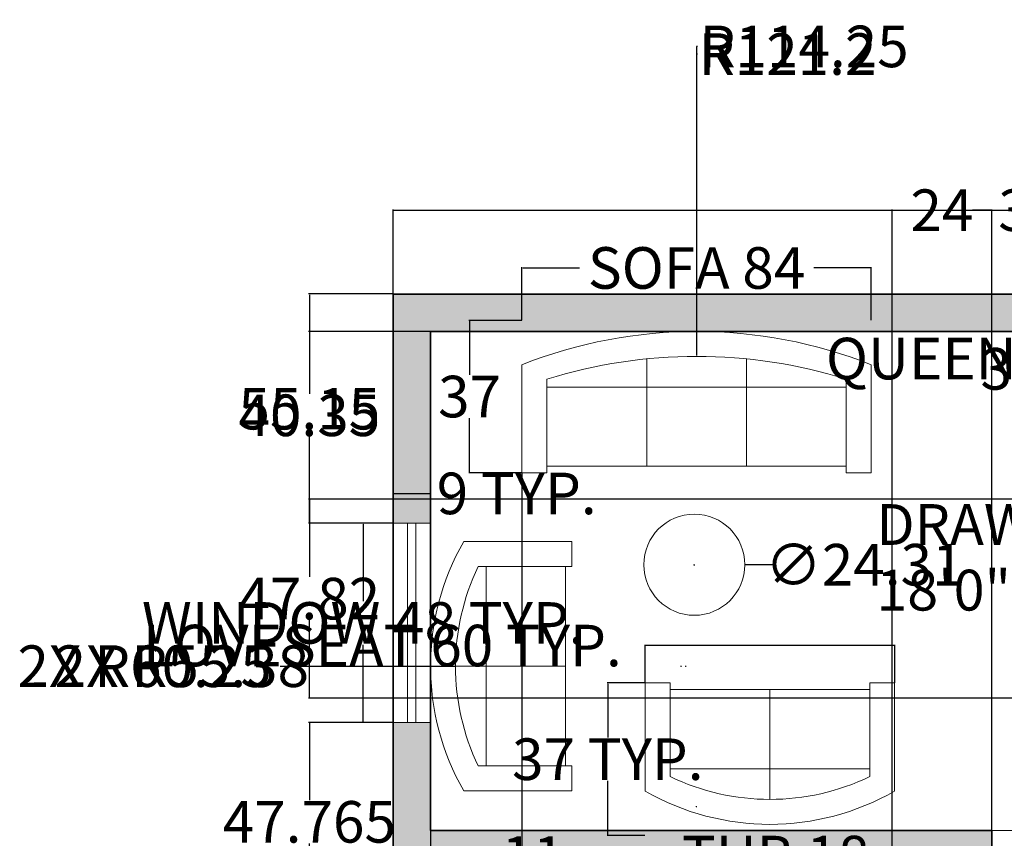
# Model space of a CAD drawing. Units: inches. Extents: x -75 to 484, y -248 to 214.
# Tile 3 of 7: x -75 to 162, y 17 to 214. Entities that reach past the tile are written whole.
import ezdxf

# ---------------------------------------------------------------- set-up
doc = ezdxf.new("R2010")
doc.units = ezdxf.units.IN
doc.header["$MEASUREMENT"] = 0
doc.linetypes.add('ACAD_ISO02W100', pattern=[15, 12, -3])
for name, color, linetype, lineweight in [('A-ANNO-DIMS', 2, 'Continuous', 18), ('A-AREA-IDEN', 7, 'Continuous', 18), ('A-FURN', 8, 'Continuous', 18), ('A-GLAZ', 4, 'Continuous', 18), ('A-WALL', 7, 'Continuous', 35), ('A-WALL-OVHD', 7, 'ACAD_ISO02W100', 18)]:
    doc.layers.add(name, color=color, linetype=linetype, lineweight=lineweight)
doc.layers.add('A-WALL-PATT', color=252, linetype='Continuous', lineweight=9, true_color=0x939598)
doc.styles.get("Standard").update_dxf_attribs({"font": 'arial.ttf'})
doc.dimstyles.get("Standard").update_dxf_attribs({"dimtxt": 10, "dimasz": 0.18, "dimexe": 0.18, "dimexo": 0.0625, "dimgap": 0.09, "dimtad": 0, "dimtih": 1, "dimtoh": 1, "dimdec": 0, "dimzin": 0, "dimdsep": 46, "dimlunit": 3, "dimtxsty": 'Standard', "dimcen": 0.09, "dimadec": 0, "dimazin": 0, "dimtfac": 1, "dimtdec": 0, "dimtofl": 0, "dimtmove": 0, "dimatfit": 3, "dimfxl": 1, "dimtolj": 1, "dimtzin": 0, "dimarcsym": 0})

# ---------------------------------------------------------------- blocks, each defined once
blk = doc.blocks.new('Sofa - Roundback 7 ft.')
for p, q in [((-12.00002, -32.4421), (-12.00003, -6.5971)), ((11.99997, -32.4421), (11.99998, -6.5971)), ((-36.000027, -34), (-36.000027, -11.4696)), ((35.99998, -34), (35.99998, -11.4696)), ((-35.999844, -13.3819), (35.9998, -13.3819)), ((-36.000027, -32.4421), (35.99998, -32.4421))]:
    blk.add_line(p, q)
for points in [[(-36.000027, -34), (-42.000027, -34), (-42.000027, -8)], [(41.99998, -8), (41.99998, -34), (35.99998, -34)]]:
    blk.add_lwpolyline(points)
for centre, radius, start, end in [((0, -114.25), 114.25, 68.43141, 111.5686), ((-0.00001, -127.1968), 121.1968, 72.72033, 107.2797)]:
    blk.add_arc(centre, radius, start, end)
blk = doc.blocks.new('Sofa - Roundback Loveseat 5 ft.')
for p, q in [((0, -32.44198), (0, -5.99998)), ((-24, -33.99998), (-24, -11.46958)), ((24.00004, -33.99998), (24.00004, -11.46958)), ((-23.9998, -13.38178), (23.99986, -13.38178)), ((-24, -32.44198), (24.00004, -32.44198))]:
    blk.add_line(p, q)
for points in [[(-24, -33.99998), (-30, -33.99998), (-30, -7.99998)], [(30.00004, -7.99998), (30.00004, -33.99998), (24.00004, -33.99998)]]:
    blk.add_lwpolyline(points)
for centre, radius, start, end in [((0, -60.24998), 60.24998, 60.13715, 119.8628), ((0, -61.38438), 55.38444, 64.32083, 115.6792)]:
    blk.add_arc(centre, radius, start, end)
blk = doc.blocks.new('WIN-48-NOM')
for p, q in [((9, 47.92), (0, 47.92)), ((3.5, 0), (3.5, 47.92)), ((5.5, 0), (5.5, 47.92)), ((0, 0), (9, 0))]:
    blk.add_line(p, q)
blk = doc.blocks.new('*D14')
at = {"layer": 'A-ANNO-DIMS', "color": 0, "lineweight": -2, "transparency": 16777216}
for p, q in [((184.84, 147.66), (179.32, 147.66)), ((179.5, 147.48), (179.5, 134.86)), ((179.5, 111.84), (179.5, 124.46)), ((184.84, 111.66), (179.32, 111.66))]:
    blk.add_line(p, q, dxfattribs=at)
at = {"layer": 'A-ANNO-DIMS', "color": 0, "transparency": 16777216}
for points in [[(179.47, 147.48), (179.53, 147.48), (179.5, 147.66)], [(179.47, 111.84), (179.53, 111.84), (179.5, 111.66)]]:
    blk.add_solid(points, dxfattribs=at)
at = {"layer": 'Defpoints', "color": 0, "transparency": 16777216}
for p in [(179.5, 147.66), (184.9, 147.66), (184.9, 111.66)]:
    blk.add_point(p, dxfattribs=at)
at = {"layer": 'A-ANNO-DIMS', "color": 0, "transparency": 16777216, "insert": (179.5, 129.66), "char_height": 10, "attachment_point": 5}
blk.add_mtext('\\A1;36 TYP.', dxfattribs=at)
blk = doc.blocks.new('*D17')
at = {"layer": 'A-ANNO-DIMS', "color": 0, "lineweight": -2, "transparency": 16777216}
for p, q in [((15.15, 92.5), (7.84, 92.5)), ((8.02, 92.32), (8.02, 73.81)), ((8.02, 44.77), (8.02, 63.28)), ((15.15, 44.59), (7.84, 44.59))]:
    blk.add_line(p, q, dxfattribs=at)
at = {"layer": 'A-ANNO-DIMS', "color": 0, "transparency": 16777216}
for points in [[(7.99, 92.32), (8.05, 92.32), (8.02, 92.5)], [(7.99, 44.77), (8.05, 44.77), (8.02, 44.59)]]:
    blk.add_solid(points, dxfattribs=at)
at = {"layer": 'Defpoints', "color": 0, "transparency": 16777216}
for p in [(8.02, 92.5), (15.21, 92.5), (15.21, 44.59)]:
    blk.add_point(p, dxfattribs=at)
at = {"layer": 'A-ANNO-DIMS', "color": 0, "transparency": 16777216, "insert": (8.02, 68.54), "char_height": 10, "attachment_point": 5}
blk.add_mtext('\\A1;WINDOW 48 TYP.', dxfattribs=at)
blk = doc.blocks.new('*D18')
at = {"layer": 'A-ANNO-DIMS', "color": 0, "lineweight": -2, "transparency": 16777216}
for p, q in [((15.21, 92.57), (15.21, 99.87)), ((15.39, 99.69), (24.03, 99.69)), ((24.21, 92.57), (24.21, 99.87)), ((24.21, 99.69), (24.39, 99.69))]:
    blk.add_line(p, q, dxfattribs=at)
at = {"layer": 'A-ANNO-DIMS', "color": 0, "transparency": 16777216}
for points in [[(15.39, 99.72), (15.39, 99.66), (15.21, 99.69)], [(24.03, 99.72), (24.03, 99.66), (24.21, 99.69)]]:
    blk.add_solid(points, dxfattribs=at)
at = {"layer": 'Defpoints', "color": 0, "transparency": 16777216}
for p in [(24.21, 99.69), (15.21, 92.5), (24.21, 92.5)]:
    blk.add_point(p, dxfattribs=at)
at = {"layer": 'A-ANNO-DIMS', "color": 0, "transparency": 16777216, "insert": (44.93, 99.69), "char_height": 10, "attachment_point": 5}
blk.add_mtext('\\A1;9 TYP.', dxfattribs=at)
blk = doc.blocks.new('*D19')
at = {"layer": 'A-ANNO-DIMS', "color": 0, "lineweight": -2, "transparency": 16777216}
for p, q in [((249.21, 132.13), (249.03, 132.13)), ((249.21, 120.19), (249.21, 132.31)), ((329.03, 132.13), (249.39, 132.13)), ((329.21, 120.19), (329.21, 132.31))]:
    blk.add_line(p, q, dxfattribs=at)
at = {"layer": 'A-ANNO-DIMS', "color": 0, "transparency": 16777216}
for points in [[(249.39, 132.16), (249.39, 132.1), (249.21, 132.13)], [(329.03, 132.16), (329.03, 132.1), (329.21, 132.13)]]:
    blk.add_solid(points, dxfattribs=at)
at = {"layer": 'Defpoints', "color": 0, "transparency": 16777216}
for p in [(249.21, 132.13), (249.21, 120.13), (329.21, 120.13)]:
    blk.add_point(p, dxfattribs=at)
at = {"layer": 'A-ANNO-DIMS', "color": 0, "transparency": 16777216, "insert": (181.53, 132.13), "char_height": 10, "attachment_point": 5}
blk.add_mtext('\\A1;QUEEN BED 80 TYP.', dxfattribs=at)
blk = doc.blocks.new('*D23')
at = {"layer": 'A-ANNO-DIMS', "color": 0, "lineweight": -2, "transparency": 16777216}
for p, q in [((75.84, 63.1), (75.66, 63.1)), ((75.84, 54.16), (75.84, 63.28)), ((135.66, 63.1), (76.02, 63.1)), ((135.84, 54.16), (135.84, 63.28))]:
    blk.add_line(p, q, dxfattribs=at)
at = {"layer": 'A-ANNO-DIMS', "color": 0, "transparency": 16777216}
for points in [[(76.02, 63.13), (76.02, 63.07), (75.84, 63.1)], [(135.66, 63.13), (135.66, 63.07), (135.84, 63.1)]]:
    blk.add_solid(points, dxfattribs=at)
at = {"layer": 'Defpoints', "color": 0, "transparency": 16777216}
for p in [(75.84, 63.1), (75.84, 54.1), (135.84, 54.1)]:
    blk.add_point(p, dxfattribs=at)
at = {"layer": 'A-ANNO-DIMS', "color": 0, "transparency": 16777216, "insert": (12.63, 63.1), "char_height": 10, "attachment_point": 5}
blk.add_mtext('\\A1;LOVESEAT 60 TYP.', dxfattribs=at)
blk = doc.blocks.new('*D24')
at = {"layer": 'A-ANNO-DIMS', "color": 0, "lineweight": -2, "transparency": 16777216}
for p, q in [((75.77, 54.1), (66.66, 54.1)), ((66.84, 53.92), (66.84, 40.97)), ((66.84, 17.61), (66.84, 30.57)), ((75.77, 17.43), (66.66, 17.43))]:
    blk.add_line(p, q, dxfattribs=at)
at = {"layer": 'A-ANNO-DIMS', "color": 0, "transparency": 16777216}
for points in [[(66.81, 53.92), (66.87, 53.92), (66.84, 54.1)], [(66.81, 17.61), (66.87, 17.61), (66.84, 17.43)]]:
    blk.add_solid(points, dxfattribs=at)
at = {"layer": 'Defpoints', "color": 0, "transparency": 16777216}
for p in [(75.84, 54.1), (66.84, 17.43), (75.84, 17.43)]:
    blk.add_point(p, dxfattribs=at)
at = {"layer": 'A-ANNO-DIMS', "color": 0, "transparency": 16777216, "insert": (66.84, 35.77), "char_height": 10, "attachment_point": 5}
blk.add_mtext('\\A1;37 TYP.', dxfattribs=at)
blk = doc.blocks.new('*D25')
at = {"layer": 'A-ANNO-DIMS', "color": 0, "lineweight": -2, "transparency": 16777216}
for p, q in [((46.2, 141.39), (46.2, 154.1)), ((130.2, 141.39), (130.2, 154.1)), ((46.38, 153.92), (60.03, 153.92)), ((130.02, 153.92), (116.37, 153.92))]:
    blk.add_line(p, q, dxfattribs=at)
at = {"layer": 'A-ANNO-DIMS', "color": 0, "transparency": 16777216}
for points in [[(46.38, 153.95), (46.38, 153.89), (46.2, 153.92)], [(130.02, 153.95), (130.02, 153.89), (130.2, 153.92)]]:
    blk.add_solid(points, dxfattribs=at)
at = {"layer": 'Defpoints', "color": 0, "transparency": 16777216}
for p in [(130.2, 153.92), (46.2, 141.32), (130.2, 141.32)]:
    blk.add_point(p, dxfattribs=at)
at = {"layer": 'A-ANNO-DIMS', "color": 0, "transparency": 16777216, "insert": (88.2, 153.92), "char_height": 10, "attachment_point": 5}
blk.add_mtext('\\A1;SOFA 84', dxfattribs=at)
blk = doc.blocks.new('*D26')
at = {"layer": 'A-ANNO-DIMS', "color": 0, "lineweight": -2, "transparency": 16777216}
for p, q in [((46.14, 141.32), (33.42, 141.32)), ((33.6, 141.14), (33.6, 128.19)), ((33.6, 104.84), (33.6, 117.79)), ((46.14, 104.66), (33.42, 104.66))]:
    blk.add_line(p, q, dxfattribs=at)
at = {"layer": 'A-ANNO-DIMS', "color": 0, "transparency": 16777216}
for points in [[(33.57, 141.14), (33.63, 141.14), (33.6, 141.32)], [(33.57, 104.84), (33.63, 104.84), (33.6, 104.66)]]:
    blk.add_solid(points, dxfattribs=at)
at = {"layer": 'Defpoints', "color": 0, "transparency": 16777216}
for p in [(33.6, 141.32), (46.2, 141.32), (46.2, 104.66)]:
    blk.add_point(p, dxfattribs=at)
at = {"layer": 'A-ANNO-DIMS', "color": 0, "transparency": 16777216, "insert": (33.6, 122.99), "char_height": 10, "attachment_point": 5}
blk.add_mtext('\\A1;37', dxfattribs=at)
blk = doc.blocks.new('*D30')
at = {"layer": 'A-ANNO-DIMS', "color": 0, "lineweight": -2, "transparency": 16777216}
for p, q in [((31.92, 9.72), (31.92, 12.43)), ((32.1, 12.25), (42.73, 12.25)), ((42.91, 9.72), (42.91, 12.43)), ((42.91, 12.25), (43.09, 12.25))]:
    blk.add_line(p, q, dxfattribs=at)
at = {"layer": 'A-ANNO-DIMS', "color": 0, "transparency": 16777216}
for points in [[(32.1, 12.28), (32.1, 12.22), (31.92, 12.25)], [(42.73, 12.28), (42.73, 12.22), (42.91, 12.25)]]:
    blk.add_solid(points, dxfattribs=at)
at = {"layer": 'Defpoints', "color": 0, "transparency": 16777216}
for p in [(42.91, 12.25), (31.92, 9.66), (42.91, 9.66)]:
    blk.add_point(p, dxfattribs=at)
at = {"layer": 'A-ANNO-DIMS', "color": 0, "transparency": 16777216, "insert": (48.9, 12.25), "char_height": 10, "attachment_point": 5}
blk.add_mtext('\\A1;11', dxfattribs=at)
blk = doc.blocks.new('*D33')
at = {"layer": 'A-ANNO-DIMS', "color": 0, "lineweight": -2, "transparency": 16777216}
for p, q in [((65.81, 9.72), (65.81, 12.53)), ((65.99, 12.35), (83.56, 12.35)), ((83.74, 9.72), (83.74, 12.53)), ((83.74, 12.35), (83.92, 12.35))]:
    blk.add_line(p, q, dxfattribs=at)
at = {"layer": 'A-ANNO-DIMS', "color": 0, "transparency": 16777216}
for points in [[(65.99, 12.38), (65.99, 12.32), (65.81, 12.35)], [(83.56, 12.38), (83.56, 12.32), (83.74, 12.35)]]:
    blk.add_solid(points, dxfattribs=at)
at = {"layer": 'Defpoints', "color": 0, "transparency": 16777216}
for p in [(83.74, 12.35), (65.81, 9.66), (83.74, 9.66)]:
    blk.add_point(p, dxfattribs=at)
at = {"layer": 'A-ANNO-DIMS', "color": 0, "transparency": 16777216, "insert": (107.22, 12.35), "char_height": 10, "attachment_point": 5}
blk.add_mtext('\\A1;TUB 18', dxfattribs=at)
blk = doc.blocks.new('*D41')
at = {"layer": 'A-ANNO-DIMS', "color": 0, "lineweight": -2, "transparency": 16777216}
for p, q in [((15.21, 147.72), (15.21, 167.99)), ((15.39, 167.81), (203.57, 167.81)), ((414.03, 167.81), (225.85, 167.81)), ((414.21, 147.72), (414.21, 167.99))]:
    blk.add_line(p, q, dxfattribs=at)
at = {"layer": 'A-ANNO-DIMS', "color": 0, "transparency": 16777216}
for points in [[(15.39, 167.84), (15.39, 167.78), (15.21, 167.81)], [(414.03, 167.84), (414.03, 167.78), (414.21, 167.81)]]:
    blk.add_solid(points, dxfattribs=at)
at = {"layer": 'Defpoints', "color": 0, "transparency": 16777216}
for p in [(414.21, 167.81), (15.21, 147.66), (414.21, 147.66)]:
    blk.add_point(p, dxfattribs=at)
at = {"layer": 'A-ANNO-DIMS', "color": 0, "transparency": 16777216, "insert": (214.71, 167.81), "char_height": 10, "attachment_point": 5}
blk.add_mtext('\\A1;399', dxfattribs=at)
blk = doc.blocks.new('*D44')
at = {"layer": 'A-ANNO-DIMS', "color": 0, "lineweight": -2, "transparency": 16777216}
for p, q in [((15.15, 147.66), (-5.12, 147.66)), ((-4.94, 147.48), (-4.94, 125.28)), ((-4.94, 92.68), (-4.94, 114.88)), ((15.15, 92.5), (-5.12, 92.5))]:
    blk.add_line(p, q, dxfattribs=at)
at = {"layer": 'A-ANNO-DIMS', "color": 0, "transparency": 16777216}
for points in [[(-4.97, 147.48), (-4.91, 147.48), (-4.94, 147.66)], [(-4.97, 92.68), (-4.91, 92.68), (-4.94, 92.5)]]:
    blk.add_solid(points, dxfattribs=at)
at = {"layer": 'Defpoints', "color": 0, "transparency": 16777216}
for p in [(15.21, 147.66), (-4.94, 92.5), (15.21, 92.5)]:
    blk.add_point(p, dxfattribs=at)
at = {"layer": 'A-ANNO-DIMS', "color": 0, "transparency": 16777216, "insert": (-4.94, 120.08), "char_height": 10, "attachment_point": 5}
blk.add_mtext('\\A1;55.15', dxfattribs=at)
blk = doc.blocks.new('*D45')
at = {"layer": 'A-ANNO-DIMS', "color": 0, "lineweight": -2, "transparency": 16777216}
for p, q in [((15.15, 44.59), (-5.12, 44.59)), ((-4.94, 44.41), (-4.94, 25.9)), ((-4.94, -3), (-4.94, 15.51)), ((15.15, -3.18), (-5.12, -3.18))]:
    blk.add_line(p, q, dxfattribs=at)
at = {"layer": 'A-ANNO-DIMS', "color": 0, "transparency": 16777216}
for points in [[(-4.97, 44.41), (-4.91, 44.41), (-4.94, 44.59)], [(-4.97, -3), (-4.91, -3), (-4.94, -3.18)]]:
    blk.add_solid(points, dxfattribs=at)
at = {"layer": 'Defpoints', "color": 0, "transparency": 16777216}
for p in [(15.21, 44.59), (-4.94, -3.18), (15.21, -3.18)]:
    blk.add_point(p, dxfattribs=at)
at = {"layer": 'A-ANNO-DIMS', "color": 0, "transparency": 16777216, "insert": (-4.94, 20.7), "char_height": 10, "attachment_point": 5}
blk.add_mtext('\\A1;47.765', dxfattribs=at)
blk = doc.blocks.new('*D50')
at = {"layer": 'A-ANNO-DIMS', "color": 0, "lineweight": -2, "transparency": 16777216}
for p, q in [((405.15, 138.66), (-5.12, 138.66)), ((-4.94, 138.48), (-4.94, 123.68)), ((-4.94, 98.48), (-4.94, 113.28)), ((405.15, 98.3), (-5.12, 98.3))]:
    blk.add_line(p, q, dxfattribs=at)
at = {"layer": 'A-ANNO-DIMS', "color": 0, "transparency": 16777216}
for points in [[(-4.97, 138.48), (-4.91, 138.48), (-4.94, 138.66)], [(-4.97, 98.48), (-4.91, 98.48), (-4.94, 98.3)]]:
    blk.add_solid(points, dxfattribs=at)
at = {"layer": 'Defpoints', "color": 0, "transparency": 16777216}
for p in [(405.21, 138.66), (-4.94, 98.3), (405.21, 98.3)]:
    blk.add_point(p, dxfattribs=at)
at = {"layer": 'A-ANNO-DIMS', "color": 0, "transparency": 16777216, "insert": (-4.94, 118.48), "char_height": 10, "attachment_point": 5}
blk.add_mtext('\\A1;40.35', dxfattribs=at)
blk = doc.blocks.new('*D51')
at = {"layer": 'A-ANNO-DIMS', "color": 0, "lineweight": -2, "transparency": 16777216}
for p, q in [((405.15, 98.3), (-5.12, 98.3)), ((-4.94, 98.12), (-4.94, 79.59)), ((-4.94, 50.66), (-4.94, 69.2)), ((405.15, 50.48), (-5.12, 50.48))]:
    blk.add_line(p, q, dxfattribs=at)
at = {"layer": 'A-ANNO-DIMS', "color": 0, "transparency": 16777216}
for points in [[(-4.97, 98.12), (-4.91, 98.12), (-4.94, 98.3)], [(-4.97, 50.66), (-4.91, 50.66), (-4.94, 50.48)]]:
    blk.add_solid(points, dxfattribs=at)
at = {"layer": 'Defpoints', "color": 0, "transparency": 16777216}
for p in [(405.21, 98.3), (-4.94, 50.48), (405.21, 50.48)]:
    blk.add_point(p, dxfattribs=at)
at = {"layer": 'A-ANNO-DIMS', "color": 0, "transparency": 16777216, "insert": (-4.94, 74.39), "char_height": 10, "attachment_point": 5}
blk.add_mtext('\\A1;47.82', dxfattribs=at)
blk = doc.blocks.new('*D54')
at = {"layer": 'A-ANNO-DIMS', "color": 0, "lineweight": -2, "transparency": 16777216}
for p, q in [((135.21, -50.28), (135.21, 167.99)), ((135.39, 167.81), (139.89, 167.81)), ((159.03, 167.81), (154.53, 167.81)), ((159.21, -50.28), (159.21, 167.99))]:
    blk.add_line(p, q, dxfattribs=at)
at = {"layer": 'A-ANNO-DIMS', "color": 0, "transparency": 16777216}
for points in [[(135.39, 167.84), (135.39, 167.78), (135.21, 167.81)], [(159.03, 167.84), (159.03, 167.78), (159.21, 167.81)]]:
    blk.add_solid(points, dxfattribs=at)
at = {"layer": 'Defpoints', "color": 0, "transparency": 16777216}
for p in [(159.21, 167.81), (135.21, -50.34), (159.21, -50.34)]:
    blk.add_point(p, dxfattribs=at)
at = {"layer": 'A-ANNO-DIMS', "color": 0, "transparency": 16777216, "insert": (147.21, 167.81), "char_height": 10, "attachment_point": 5}
blk.add_mtext('\\A1;24', dxfattribs=at)
blk = doc.blocks.new('*D76')
at = {"layer": 'A-ANNO-DIMS', "color": 0, "lineweight": -2, "transparency": 16777216}
for p, q in [((24.21, 138.59), (24.21, -241.67)), ((46.2, 104.59), (46.2, -241.67)), ((24.39, -241.49), (46.02, -241.49)), ((46.2, -241.49), (46.38, -241.49))]:
    blk.add_line(p, q, dxfattribs=at)
at = {"layer": 'A-ANNO-DIMS', "color": 0, "transparency": 16777216}
for points in [[(24.39, -241.46), (24.39, -241.52), (24.21, -241.49)], [(46.02, -241.46), (46.02, -241.52), (46.2, -241.49)]]:
    blk.add_solid(points, dxfattribs=at)
at = {"layer": 'Defpoints', "color": 0, "transparency": 16777216}
for p in [(24.21, 138.66), (46.2, 104.66), (46.2, -241.49)]:
    blk.add_point(p, dxfattribs=at)
at = {"layer": 'A-ANNO-DIMS', "color": 0, "transparency": 16777216, "insert": (63.44, -241.49), "char_height": 10, "attachment_point": 5}
blk.add_mtext('\\A1;21.99', dxfattribs=at)
blk = doc.blocks.new('*D77')
at = {"layer": 'A-ANNO-DIMS', "color": 0, "lineweight": -2, "transparency": 16777216}
for p, q in [((159.21, -53.28), (159.21, 167.99)), ((159.39, 167.81), (160.83, 167.81)), ((196.22, 167.81), (194.77, 167.81)), ((196.4, -54.9), (196.4, 167.99))]:
    blk.add_line(p, q, dxfattribs=at)
at = {"layer": 'A-ANNO-DIMS', "color": 0, "transparency": 16777216}
for points in [[(159.39, 167.84), (159.39, 167.78), (159.21, 167.81)], [(196.22, 167.84), (196.22, 167.78), (196.4, 167.81)]]:
    blk.add_solid(points, dxfattribs=at)
at = {"layer": 'Defpoints', "color": 0, "transparency": 16777216}
for p in [(196.4, 167.81), (159.21, -53.34), (196.4, -54.96)]:
    blk.add_point(p, dxfattribs=at)
at = {"layer": 'A-ANNO-DIMS', "color": 0, "transparency": 16777216, "insert": (177.8, 167.81), "char_height": 10, "attachment_point": 5}
blk.add_mtext('\\A1;37.19', dxfattribs=at)
blk = doc.blocks.new('*D81')
at = {"layer": 'A-ANNO-DIMS', "color": 0, "lineweight": -2, "transparency": 16777216}
for p, q in [((159.21, 18.72), (159.21, 167.99)), ((159.39, 167.81), (193.42, 167.81)), ((240.03, 167.81), (206, 167.81)), ((240.21, 18.72), (240.21, 167.99))]:
    blk.add_line(p, q, dxfattribs=at)
at = {"layer": 'A-ANNO-DIMS', "color": 0, "transparency": 16777216}
for points in [[(159.39, 167.84), (159.39, 167.78), (159.21, 167.81)], [(240.03, 167.84), (240.03, 167.78), (240.21, 167.81)]]:
    blk.add_solid(points, dxfattribs=at)
at = {"layer": 'Defpoints', "color": 0, "transparency": 16777216}
for p in [(240.21, 167.81), (159.21, 18.66), (240.21, 18.66)]:
    blk.add_point(p, dxfattribs=at)
at = {"layer": 'A-ANNO-DIMS', "color": 0, "transparency": 16777216, "insert": (199.71, 167.81), "char_height": 10, "attachment_point": 5}
blk.add_mtext('\\A1;81', dxfattribs=at)
blk = doc.blocks.new('*D83')
at = {"layer": 'A-ANNO-DIMS', "color": 0, "lineweight": -2, "transparency": 16777216}
for p, q in [((87.56, 82.54), (87.74, 82.54)), ((87.65, 82.45), (87.65, 82.63)), ((107.1, 82.54), (99.99, 82.54))]:
    blk.add_line(p, q, dxfattribs=at)
at = {"layer": 'A-ANNO-DIMS', "color": 0, "transparency": 16777216}
blk.add_solid([(99.99, 82.57), (99.99, 82.51), (99.81, 82.54)], dxfattribs=at)
at = {"layer": 'Defpoints', "color": 0, "transparency": 16777216}
for p in [(75.5, 82.54), (99.81, 82.54)]:
    blk.add_point(p, dxfattribs=at)
at = {"layer": 'A-ANNO-DIMS', "color": 0, "transparency": 16777216, "insert": (128.54, 82.54), "char_height": 10, "attachment_point": 5}
blk.add_mtext('\\A1;∅24.31', dxfattribs=at)
blk = doc.blocks.new('*D84')
at = {"layer": 'A-ANNO-DIMS', "color": 0, "lineweight": -2, "transparency": 16777216}
for p, q in [((88.38, 205.37), (88.2, 205.37)), ((88.2, 205.37), (88.2, 132.84)), ((88.11, 11.46), (88.29, 11.46)), ((88.2, 11.37), (88.2, 11.55))]:
    blk.add_line(p, q, dxfattribs=at)
at = {"layer": 'A-ANNO-DIMS', "color": 0, "transparency": 16777216}
blk.add_solid([(88.17, 132.84), (88.23, 132.84), (88.2, 132.66)], dxfattribs=at)
at = {"layer": 'Defpoints', "color": 0, "transparency": 16777216}
for p in [(88.2, 132.66), (88.2, 11.46)]:
    blk.add_point(p, dxfattribs=at)
at = {"layer": 'A-ANNO-DIMS', "color": 0, "transparency": 16777216, "insert": (110.08, 205.37), "char_height": 10, "attachment_point": 5}
blk.add_mtext('\\A1;R121.2', dxfattribs=at)
blk = doc.blocks.new('*D85')
at = {"layer": 'A-ANNO-DIMS', "color": 0, "lineweight": -2, "transparency": 16777216}
for p, q in [((88.38, 207.21), (88.2, 207.21)), ((88.2, 207.21), (88.2, 138.84)), ((88.11, 24.41), (88.29, 24.41)), ((88.2, 24.32), (88.2, 24.5))]:
    blk.add_line(p, q, dxfattribs=at)
at = {"layer": 'A-ANNO-DIMS', "color": 0, "transparency": 16777216}
blk.add_solid([(88.17, 138.84), (88.23, 138.84), (88.2, 138.66)], dxfattribs=at)
at = {"layer": 'Defpoints', "color": 0, "transparency": 16777216}
for p in [(88.2, 138.66), (88.2, 24.41)]:
    blk.add_point(p, dxfattribs=at)
at = {"layer": 'A-ANNO-DIMS', "color": 0, "transparency": 16777216, "insert": (114.05, 207.21), "char_height": 10, "attachment_point": 5}
blk.add_mtext('\\A1;R114.25', dxfattribs=at)
blk = doc.blocks.new('*D86')
at = {"layer": 'A-ANNO-DIMS', "color": 0, "lineweight": -2, "transparency": 16777216}
for p, q in [((-11.94, 58.14), (24.03, 58.14)), ((84.37, 58.14), (84.55, 58.14)), ((84.46, 58.05), (84.46, 58.23))]:
    blk.add_line(p, q, dxfattribs=at)
at = {"layer": 'A-ANNO-DIMS', "color": 0, "transparency": 16777216}
blk.add_solid([(24.03, 58.17), (24.03, 58.11), (24.21, 58.14)], dxfattribs=at)
at = {"layer": 'Defpoints', "color": 0, "transparency": 16777216}
for p in [(24.21, 58.14), (84.46, 58.14)]:
    blk.add_point(p, dxfattribs=at)
at = {"layer": 'A-ANNO-DIMS', "color": 0, "transparency": 16777216, "insert": (-44.55, 58.14), "char_height": 10, "attachment_point": 5}
blk.add_mtext('\\A1;2X R60.25', dxfattribs=at)
blk = doc.blocks.new('*D87')
at = {"layer": 'A-ANNO-DIMS', "color": 0, "lineweight": -2, "transparency": 16777216}
for p, q in [((-3.02, 58.14), (30.03, 58.14)), ((85.5, 58.14), (85.68, 58.14)), ((85.59, 58.05), (85.59, 58.23))]:
    blk.add_line(p, q, dxfattribs=at)
at = {"layer": 'A-ANNO-DIMS', "color": 0, "transparency": 16777216}
blk.add_solid([(30.03, 58.17), (30.03, 58.11), (30.21, 58.14)], dxfattribs=at)
at = {"layer": 'Defpoints', "color": 0, "transparency": 16777216}
for p in [(30.21, 58.14), (85.59, 58.14)]:
    blk.add_point(p, dxfattribs=at)
at = {"layer": 'A-ANNO-DIMS', "color": 0, "transparency": 16777216, "insert": (-35.61, 58.14), "char_height": 10, "attachment_point": 5}
blk.add_mtext('\\A1;2X R55.38', dxfattribs=at)

msp = doc.modelspace()

# ---------------------------------------------------------------- hatches: boundary and pattern name
at = {"layer": 'A-WALL-PATT'}
h = msp.add_hatch(color=256, dxfattribs=at)
h.dxf.hatch_style = 1
h.paths.add_polyline_path([(184.9004, 147.6567), (15.2094, 147.6567), (15.2094, 92.5031), (24.2094, 92.5031), (24.2094, 138.6567), (186.0436, 138.6567, -0.06325422)])
h.paths.add_polyline_path([(414.2094, 147.6567), (249.2094, 147.6567), (220.9004, 147.6567), (220.9004, 138.6567), (240.2094, 138.6567), (240.2094, 18.6567), (240.2094, 9.6567), (249.2094, 9.6567), (249.2094, 45.6567), (249.2094, 138.6567), (405.2094, 138.6567), (405.2094, 98.3029), (414.2094, 98.3029)])
h.paths.add_polyline_path([(159.2094, 18.6567), (24.2094, 18.6567), (24.2094, 44.5861), (15.2094, 44.5861), (15.2094, 9.6567), (15.2094, -3.1791), (24.2094, -3.1791), (24.2094, 9.6567), (132.2094, 9.6567), (132.2094, -50.3433), (83.7394, -50.3433), (83.7394, -53.3433), (132.2094, -53.3433), (159.2094, -53.3433), (159.2094, -50.3433), (135.2094, -50.3433), (135.2094, 9.6567), (159.2094, 9.6567)])
h.paths.add_polyline_path([(53.8898, -50.3433), (24.2094, -50.3433), (24.2094, -27.303), (15.2094, -27.303), (15.2094, -50.3433), (15.2094, -53.3433), (15.2094, -74.0487), (24.2094, -74.0487), (24.2094, -53.3433), (53.7394, -53.3433, -0.02504709)])
h.paths.add_polyline_path([(24.2094, -121.9657), (15.2094, -121.9657), (15.2094, -212.3433), (15.2094, -221.3433), (24.2094, -221.3433), (84.3017, -221.3433), (84.3017, -212.3433), (24.2094, -212.3433)])
h.paths.add_polyline_path([(414.2094, -155.3433), (414.2094, -53.3433), (414.2094, -50.3433), (414.2094, -36.8417), (405.2094, -36.8417), (405.2094, -50.3433), (309.2094, -50.3433), (309.2094, 16.0463), (324.2573, 16.0463), (324.2573, 18.6567), (284.0663, 18.6567, -0.06325422), (285.2094, 9.6567), (306.2094, 9.6567), (306.2094, -50.3433), (285.2094, -50.3433), (285.2094, -53.3433), (309.2094, -53.3433), (405.2094, -53.3433), (405.2094, -212.3433), (293.2094, -212.3433), (293.2094, -158.3433), (293.2094, -145.3433), (300.0339, -145.3433), (300.0339, -142.3433), (285.2094, -142.3433), (159.2094, -142.3433), (159.2094, -89.3433, -0.02086055), (156.2094, -89.218), (156.2094, -212.3433), (131.9001, -212.3433), (131.9001, -221.3433), (156.2094, -221.3433), (165.2094, -221.3433), (285.2094, -221.3433), (288.6713, -221.3433), (293.2094, -221.3433), (405.2094, -221.3433), (414.2094, -221.3433)])
h.paths.add_polyline_path([(165.2094, -212.3433), (165.2094, -151.3433), (285.2094, -151.3433), (285.2094, -212.3433)], flags=16)
h.paths.add_polyline_path([(189.462, -195.5437), (182.159, -190.2838, -0.23606798), (182.5164, -188.0765), (181.7049, -187.4921), (185.5037, -182.2177), (184.648, -181.6013, -0.04492589), (180.0821, -186.3232), (179.2706, -185.7388), (189.206, -171.9443), (190.0174, -172.5287, -0.04492589), (186.9857, -178.3556), (187.8415, -178.9719), (191.6403, -173.6976), (192.4517, -174.282, -0.23606798), (194.432, -173.2435), (201.735, -178.5034, -0.23606798), (201.3776, -180.7107), (202.189, -181.2952, -0.11764706), (192.2537, -195.0897), (191.4423, -194.5053, -0.23606798)], flags=0)
h.paths.add_polyline_path([(253.751, -177.9543), (254.5293, -177.3263, -0.23606798), (254.0517, -175.1419), (261.056, -169.4904, -0.23606798), (263.0902, -170.419), (263.8684, -169.7911), (267.95, -174.8498), (268.7708, -174.1875, -0.04492589), (265.425, -168.5352), (266.2032, -167.9073), (276.8782, -181.1378), (276.0999, -181.7657, -0.04492589), (271.2826, -177.3006), (270.4618, -177.9629), (274.5434, -183.0216), (273.7651, -183.6495, -0.23606798), (274.2427, -185.834), (267.2383, -191.4854, -0.23606798), (265.2042, -190.5568), (264.4259, -191.1848, -0.11764706)], flags=0)
h.paths.add_polyline_path([(405.2094, -142.3433), (336.0339, -142.3433, -0.02086055), (335.9087, -145.3433), (405.2094, -145.3433)], flags=17)
h.paths.add_polyline_path([(414.2094, 50.4831), (405.2094, 50.4831), (405.2094, 18.6567), (354.2573, 18.6567, -0.02178446), (354.1435, 16.0463), (405.2094, 16.0463), (405.2094, -14.6494), (414.2094, -14.6494), (414.2094, 9.6567)])
h.paths.add_polyline_path([(200.2091, -179.9247), (255.2702, -179.9247), (255.2702, -168.0448), (200.2091, -168.0448)], flags=8)
h.paths.add_polyline_path([(200.2352, -167.6036), (249.7883, -167.6036), (249.7883, -155.8804), (200.2352, -155.8804)], flags=8)

# ---------------------------------------------------------------- linework, layer by layer
at = {"layer": 'A-FURN'}
msp.add_circle((87.6517, 82.5399), 12.1561, dxfattribs=at)
at = {"layer": 'A-GLAZ'}
msp.add_line((19.7094, 92.5031), (24.2094, 92.5031), dxfattribs=at)
at = {"layer": 'A-WALL'}
msp.add_line((159.2094, 9.6567), (159.2094, 18.6567), dxfattribs=at)
for points in [[(249.2094, 147.6567), (15.2094, 147.6567), (15.2094, 9.6567)], [(186.0436, 138.6567), (24.2094, 138.6567), (24.2094, 18.6567), (159.2094, 18.6567)]]:
    msp.add_lwpolyline(points, dxfattribs=at)
at = {"layer": 'A-WALL-OVHD'}
msp.add_line((159.2094, 18.6567), (240.2094, 18.6567), dxfattribs=at)

# ---------------------------------------------------------------- block references
at = {"layer": 'A-FURN'}
msp.add_blockref('Sofa - Roundback 7 ft.', (88.1999, 138.6567), dxfattribs=at)
for p, rotation in [((24.2094, 58.1364), 90.00000000000003), ((105.8352, 20.1002), 180)]:
    msp.add_blockref('Sofa - Roundback Loveseat 5 ft.', p, dxfattribs=dict(at, rotation=rotation))
at = {"layer": 'A-GLAZ'}
msp.add_blockref('WIN-48-NOM', (15.2094, 44.5861), dxfattribs=at)

# ---------------------------------------------------------------- texts
at = {"layer": 'A-AREA-IDEN'}
for s, height, p in [('DRAWING', 9.82058, (131.4281, 87.2987)), ('18\'0"X10\'0"', 9.820584, (131.4281, 71.5228))]:
    msp.add_text(s, height=height, dxfattribs=at).set_placement(p)

# ---------------------------------------------------------------- dimensions: what is measured, and where the dimension line sits
at = {"layer": 'A-ANNO-DIMS'}
for center, mpoint, override, picture, middle in [((88.1999, 24.4067), (88.2, 138.6567), {"dimdec": 2, "dimlfac": 1, "dimrnd": 0, "dimzin": 0, "dimdsep": 46, "dimlunit": 2}, '*D85', (114.0499, 207.2067)), ((88.1998, 11.4599), (88.2, 132.6567), {"dimdec": 1, "dimlfac": 1, "dimrnd": 0, "dimzin": 0, "dimdsep": 46, "dimlunit": 2}, '*D84', (110.0765, 205.3748))]:
    dim = msp.add_radius_dim(center=center, mpoint=mpoint, dimstyle='Standard', override=override, dxfattribs=at)
    dim.commit()
    dim.dimension.update_dxf_attribs({"geometry": picture, "text_midpoint": middle, "dimtype": 164})
for base, p1, p2, override, picture, middle in [((414.2094, 167.8067), (15.2094, 147.6567), (414.2094, 147.6567), {"dimdec": 0, "dimlfac": 1, "dimrnd": 0, "dimzin": 0, "dimdsep": 46, "dimlunit": 2}, '*D41', (214.7094, 167.8067)), ((159.2094, 167.8067), (135.2094, -50.3433), (159.2094, -50.3433), {"dimdec": 0, "dimlfac": 1, "dimrnd": 0, "dimzin": 0, "dimdsep": 46, "dimlunit": 2}, '*D54', (147.2094, 167.8067)), ((196.3986, 167.8067), (159.2094, -53.3433), (196.3986, -54.9627), {"dimdec": 2, "dimlfac": 1, "dimrnd": 0, "dimzin": 0, "dimdsep": 46, "dimlunit": 2}, '*D77', (177.804, 167.8067)), ((240.2094, 167.8067), (159.2094, 18.6567), (240.2094, 18.6567), {"dimdec": 0, "dimlfac": 1, "dimrnd": 0, "dimzin": 0, "dimdsep": 46, "dimlunit": 2}, '*D81', (199.7094, 167.8067)), ((46.1998, -241.4933), (24.2094, 138.6567), (46.1998, 104.6567), {"dimdec": 2, "dimlfac": 1, "dimrnd": 0, "dimzin": 0, "dimdsep": 46, "dimlunit": 2}, '*D76', (63.4378, -241.4933)), ((42.9065, 12.2512), (31.915, 9.6567), (42.9065, 9.6567), {"dimdec": 0, "dimlfac": 1, "dimrnd": 0, "dimzin": 0, "dimdsep": 46, "dimlunit": 2}, '*D30', (48.903, 12.2512))]:
    dim = msp.add_linear_dim(base=base, p1=p1, p2=p2, dimstyle='Standard', override=override, dxfattribs=at)
    dim.commit()
    dim.dimension.update_dxf_attribs({"geometry": picture, "text_midpoint": middle})
for base, p1, p2, text, picture, middle in [((130.1998, 153.9234), (46.1998, 141.3234), (130.1998, 141.3234), 'SOFA <>', '*D25', (88.1998, 153.9234)), ((24.2094, 99.6906), (15.2094, 92.5031), (24.2094, 92.5031), '<> TYP.', '*D18', (44.933, 99.6906)), ((83.7394, 12.3454), (65.8148, 9.6567), (83.7394, 9.6567), 'TUB <>', '*D33', (107.2188, 12.3454))]:
    dim = msp.add_linear_dim(base=base, p1=p1, p2=p2, text=text, dimstyle='Standard', override={"dimdec": 0, "dimlfac": 1, "dimrnd": 0, "dimzin": 0, "dimdsep": 46, "dimlunit": 2}, dxfattribs=at)
    dim.commit()
    dim.dimension.update_dxf_attribs({"geometry": picture, "text_midpoint": middle})
for base, p1, p2, angle, text, picture, middle in [((249.2094, 132.1301), (329.2094, 120.1301), (249.2094, 120.1301), 180, 'QUEEN BED <> TYP.', '*D19', (181.5281, 132.1301)), ((179.5004, 147.6567), (184.9004, 111.6567), (184.9004, 147.6567), 90, '<> TYP.', '*D14', (179.5004, 129.6567)), ((8.0219, 92.5031), (15.2094, 44.5861), (15.2094, 92.5031), 90, 'WINDOW <> TYP.', '*D17', (8.0219, 68.5446)), ((75.8352, 63.1002), (135.8352, 54.1002), (75.8352, 54.1002), 180, 'LOVESEAT <> TYP.', '*D23', (12.6286, 63.1002)), ((66.8352, 17.4335), (75.8352, 54.1002), (75.8352, 17.4335), 270, '<> TYP.', '*D24', (66.8352, 35.7668))]:
    dim = msp.add_linear_dim(base=base, p1=p1, p2=p2, angle=angle, text=text, dimstyle='Standard', override={"dimdec": 0, "dimlfac": 1, "dimrnd": 0, "dimzin": 0, "dimdsep": 46, "dimlunit": 2}, dxfattribs=at)
    dim.commit()
    dim.dimension.update_dxf_attribs({"geometry": picture, "text_midpoint": middle})
for base, p1, p2, override, picture, middle in [((-4.9406, 92.5031), (15.2094, 147.6567), (15.2094, 92.5031), {"dimdec": 2, "dimlfac": 1, "dimrnd": 0, "dimzin": 0, "dimdsep": 46, "dimlunit": 2}, '*D44', (-4.9406, 120.0799)), ((33.5998, 141.3234), (46.1998, 104.6567), (46.1998, 141.3234), {"dimdec": 0, "dimlfac": 1, "dimrnd": 0, "dimzin": 0, "dimdsep": 46, "dimlunit": 2}, '*D26', (33.5998, 122.9901)), ((-4.9406, 98.3029), (405.2094, 138.6567), (405.2094, 98.3029), {"dimdec": 2, "dimlfac": 1, "dimrnd": 0, "dimzin": 0, "dimdsep": 46, "dimlunit": 2}, '*D50', (-4.9406, 118.4798)), ((-4.9406, 50.4831), (405.2094, 98.3029), (405.2094, 50.4831), {"dimdec": 2, "dimlfac": 1, "dimrnd": 0, "dimzin": 0, "dimdsep": 46, "dimlunit": 2}, '*D51', (-4.9406, 74.393)), ((-4.9406, -3.1791), (15.2094, 44.5861), (15.2094, -3.1791), {"dimdec": 3, "dimlfac": 1, "dimrnd": 0, "dimzin": 0, "dimdsep": 46, "dimlunit": 2}, '*D45', (-4.9406, 20.7035))]:
    dim = msp.add_linear_dim(base=base, p1=p1, p2=p2, angle=90, dimstyle='Standard', override=override, dxfattribs=at)
    dim.commit()
    dim.dimension.update_dxf_attribs({"geometry": picture, "text_midpoint": middle})
dim = msp.add_diameter_dim_2p(p1=(75.4956, 82.5397), p2=(99.8078, 82.54), dimstyle='Standard', override={"dimdec": 2, "dimlfac": 1, "dimrnd": 0, "dimzin": 0, "dimdsep": 46, "dimlunit": 2}, dxfattribs=at)
dim.commit()
dim.dimension.update_dxf_attribs({"geometry": '*D83', "text_midpoint": (107.1014, 82.5401), "dimtype": 163})
for center, mpoint, picture, middle in [((84.4594, 58.1364), (24.2094, 58.136), '*D86', (-11.9406, 58.1358)), ((85.5938, 58.1364), (30.2093, 58.136), '*D87', (-3.0213, 58.1358))]:
    dim = msp.add_radius_dim(center=center, mpoint=mpoint, text='2X <>', dimstyle='Standard', override={"dimdec": 2, "dimlfac": 1, "dimrnd": 0, "dimzin": 0, "dimdsep": 46, "dimlunit": 2}, dxfattribs=at)
    dim.commit()
    dim.dimension.update_dxf_attribs({"geometry": picture, "text_midpoint": middle, "dimtype": 164})

doc.saveas('drawing.dxf')
